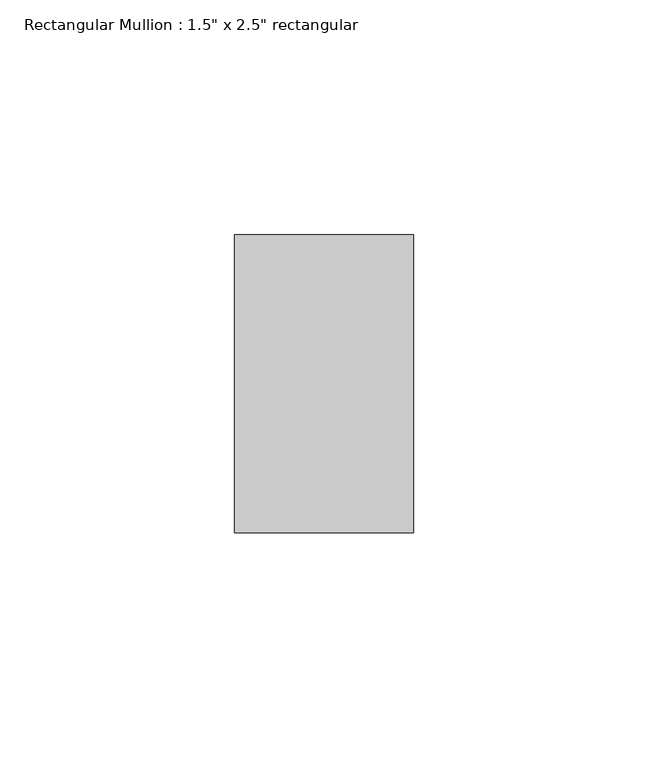
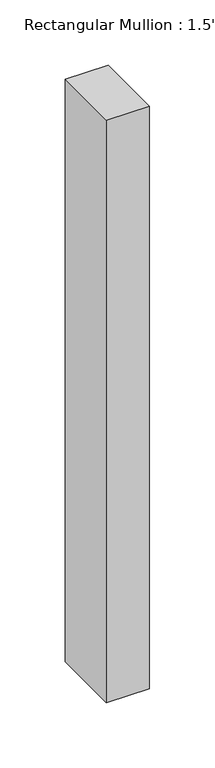
"""IFC4 building model written with IfcOpenShell, lengths in millimetres: member geometry."""

from ifc_helpers import new_model, si_unit, frame, origin, place, context, project, spatial, polyline, outline, extrude, source, transform, mapped, element, save


def member_3578a4a6(model_context):
    return source(origin(), model_context, "Body", "SweptSolid", [
        extrude(outline(polyline([(19.05, 31.75), (19.05, -31.75), (-19.05, -31.75), (-19.05, 31.75), (19.05, 31.75)])), frame((0.0, 0.0, -546.1), z_axis=(0.0, 0.0, 1.0), x_axis=(1.0, 0.0, 0.0)), (0.0, 0.0, 1.0), 546.1),
    ])


if __name__ == "__main__":
    model = new_model("IFC4")
    model_context = context("Model", 3, world=origin())
    ifc_project = project(units=[si_unit("LENGTHUNIT", "METRE", prefix="MILLI")], contexts=[model_context])
    site = spatial("IfcSite", under=ifc_project)
    building = spatial("IfcBuilding", under=site)
    placement = place(None, origin())
    member_shape = member_3578a4a6(model_context)
    element("IfcMember", 1, ObjectType="Rectangular Mullion : 1.5\" x 2.5\" rectangular", at=placement, inside=building, context=model_context, shape_type="MappedRepresentation", body=[
        mapped(member_shape, transform((0.0, 0.0, 0.0), x_axis=(1.0, 0.0, 0.0), y_axis=(0.0, 1.0, 0.0), z_axis=(0.0, 0.0, 1.0))),
    ])
    save(model, "model.ifc")

# Revit data of these elements
# Type "Rectangular Mullion : 1.5\" x 2.5\" rectangular"
#   built-in parameter 1007304 = 0.208333 (stored number, unit not read)
#   built-in parameter 1007301 = 0.0625 (stored number, unit not read)
#   built-in parameter 1007300 = 0.0625 (stored number, unit not read)
# Element 1 (IfcMember, "Rectangular Mullion : 1.5\" x 2.5\" rectangular")
#   Materials on its faces: "Aluminum"
# Materials
#   "Aluminum": class "Metal", colour RGB 247 247 247, transparency 0, Description = "Aluminum 6061", Cost = 0
